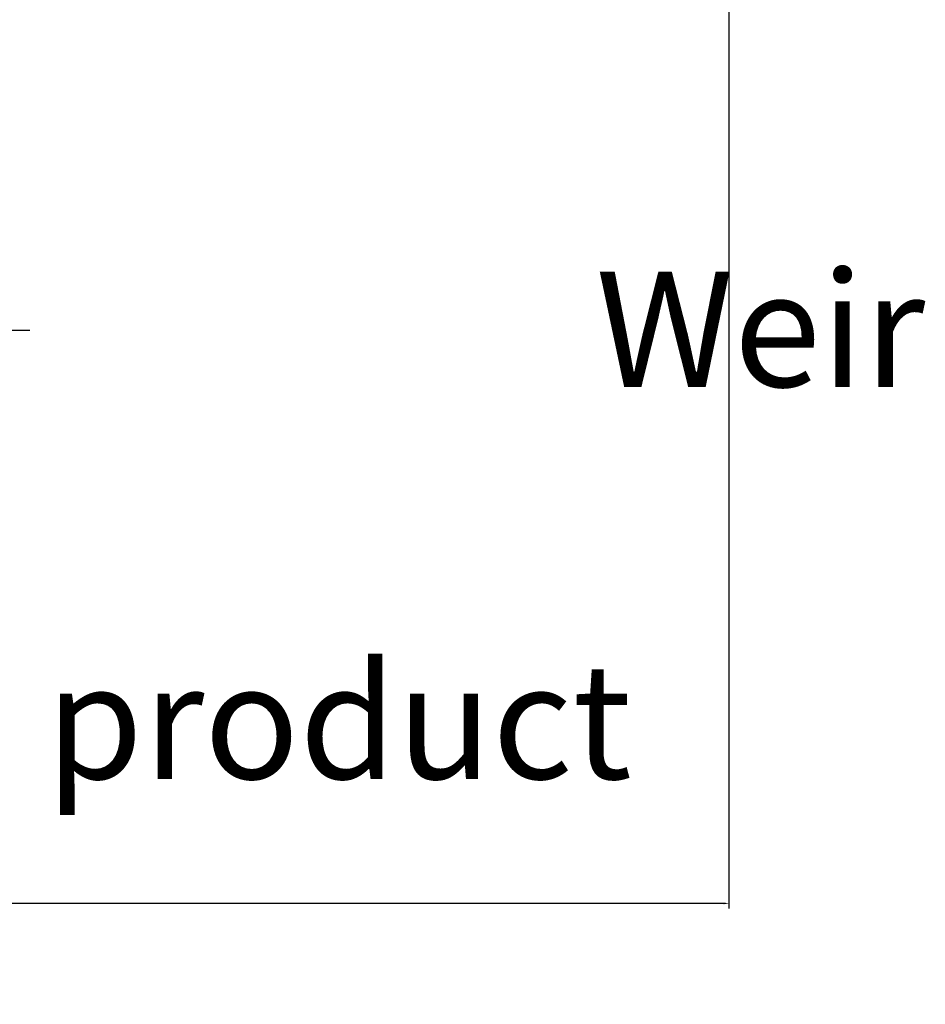
# Model space of a CAD drawing. Units: inches. Extents: x -12 to 334, y -10 to 186.
# Tile 69 of 77: x 257 to 288, y 11 to 45. Entities that reach past the tile are written whole.
import ezdxf
from ezdxf import colors
from ezdxf.entities.mleader import LeaderData, LeaderLine
from ezdxf.math import Vec2, Vec3

# ---------------------------------------------------------------- set-up
doc = ezdxf.new("R2010")
doc.units = ezdxf.units.IN
doc.header["$MEASUREMENT"] = 0
doc.layers.add('M-ANNO-TEXT', color=3, linetype='Continuous', lineweight=25)
doc.layers.add('M-DIMS', color=2, linetype='Continuous', lineweight=18)
doc.styles.get("Standard").update_dxf_attribs({"font": 'arial.ttf'})
doc.dimstyles.get("Standard").update_dxf_attribs({"dimtxt": 0.18, "dimasz": 0.18, "dimexe": 0.18, "dimexo": 0.0625, "dimgap": 0.09, "dimtad": 0, "dimtih": 1, "dimtoh": 1, "dimdec": 4, "dimzin": 0, "dimdsep": 46, "dimtxsty": 'Standard', "dimcen": 0.09, "dimadec": 0, "dimazin": 0, "dimtfac": 1, "dimtdec": 4, "dimtofl": 0, "dimtmove": 0, "dimatfit": 3, "dimfxl": 1, "dimtolj": 1, "dimtzin": 0, "dimarcsym": 0})

# ---------------------------------------------------------------- blocks, each defined once
blk = doc.blocks.new('*D1')
at = {"layer": 'Defpoints', "color": 0, "transparency": 16777216}
for p in [(281.426, 91.899), (3.376, 80.692), (281.426, 14.304)]:
    blk.add_point(p, dxfattribs=at)
at = {"layer": 'M-DIMS', "color": 0, "lineweight": -2, "transparency": 16777216}
for p, q in [((281.426, 91.836), (281.426, 14.124)), ((3.376, 80.629), (3.376, 14.124)), ((3.556, 14.304), (141.935, 14.304)), ((281.246, 14.304), (142.867, 14.304))]:
    blk.add_line(p, q, dxfattribs=at)
at = {"layer": 'M-DIMS', "color": 0, "transparency": 16777216}
for points in [[(3.556, 14.334), (3.556, 14.274), (3.376, 14.304)], [(281.246, 14.334), (281.246, 14.274), (281.426, 14.304)]]:
    blk.add_solid(points, dxfattribs=at)
at = {"layer": 'M-DIMS', "color": 0, "transparency": 16777216, "insert": (142.401, 14.304), "char_height": 0.18, "attachment_point": 5}
blk.add_mtext('\\A1;278.05', dxfattribs=at)

msp = doc.modelspace()

# ---------------------------------------------------------------- dimensions: what is measured, and where the dimension line sits
at = {"layer": 'M-DIMS'}
dim = msp.add_linear_dim(base=(281.4256, 14.3041), p1=(3.3765, 80.6915), p2=(281.4256, 91.8988), dimstyle='Standard', override={"dimdec": 2, "dimlfac": 1, "dimrnd": 0, "dimzin": 0, "dimdsep": 46, "dimlunit": 2}, dxfattribs=at)
dim.commit()
dim.dimension.update_dxf_attribs({"geometry": '*D1', "text_midpoint": (142.401, 14.3041)})

# ---------------------------------------------------------------- leaders
at = {"layer": 'M-ANNO-TEXT'}
ml = msp.add_multileader_mtext('Standard', dxfattribs=at)
ml.set_content('^I^IWeir', color=256)
ml.set_leader_properties()
ml.build(insert=Vec2(0, 0))
ml.multileader.update_dxf_attribs({"dogleg_length": 0.36, "arrow_head_size": 0.7})
ctx = ml.context
ctx.base_point, ctx.arrow_head_size, ctx.landing_gap_size, ctx.plane_origin = Vec3(257.1525, 34.1955), 0.7, 0.09, Vec3(247.9354, 49.9015)
notes = []
notes.append((ctx, [(0, (1, 1, 0), (255.3593, 34.1955), (1, 0), 1.7932, [(0, [(247.9354, 49.9015)], 0, [])])]))
ctx.mtext.insert, ctx.mtext.flow_direction = Vec3(257.2425, 36.2283), 5
ml = msp.add_multileader_mtext('Standard', dxfattribs=at)
ml.set_content('Bottom product', color=256)
ml.set_leader_properties()
ml.build(insert=Vec2(0, 0))
ml.multileader.update_dxf_attribs({"dogleg_length": 0.36, "arrow_head_size": 0.7})
ctx = ml.context
ctx.base_point, ctx.arrow_head_size, ctx.landing_gap_size, ctx.plane_origin = Vec3(237.0261, 20.0676), 0.7, 0.09, Vec3(227.5761, 30.8541)
notes.append((ctx, [(0, (1, 1, 0), (233.8037, 20.0676), (1, 0), 3.2224, [(0, [(227.5761, 30.8541)], 0, [])])]))
ctx.mtext.insert, ctx.mtext.flow_direction = Vec3(237.1161, 22.6228), 5
for ctx, leaders in notes:
    for number, flags, end, landing, length, lines in leaders:
        leader = LeaderData()
        leader.index, (leader.has_last_leader_line, leader.has_dogleg_vector, leader.attachment_direction) = number, flags
        leader.last_leader_point, leader.dogleg_vector, leader.dogleg_length = Vec3(end), Vec3(landing), length
        for number, points, colour, breaks in lines:
            line = LeaderLine()
            line.index, line.vertices, line.color, line.breaks = number, Vec3.list(points), colors.encode_raw_color(colour), breaks
            leader.lines.append(line)
        ctx.leaders.append(leader)

doc.saveas('drawing.dxf')
